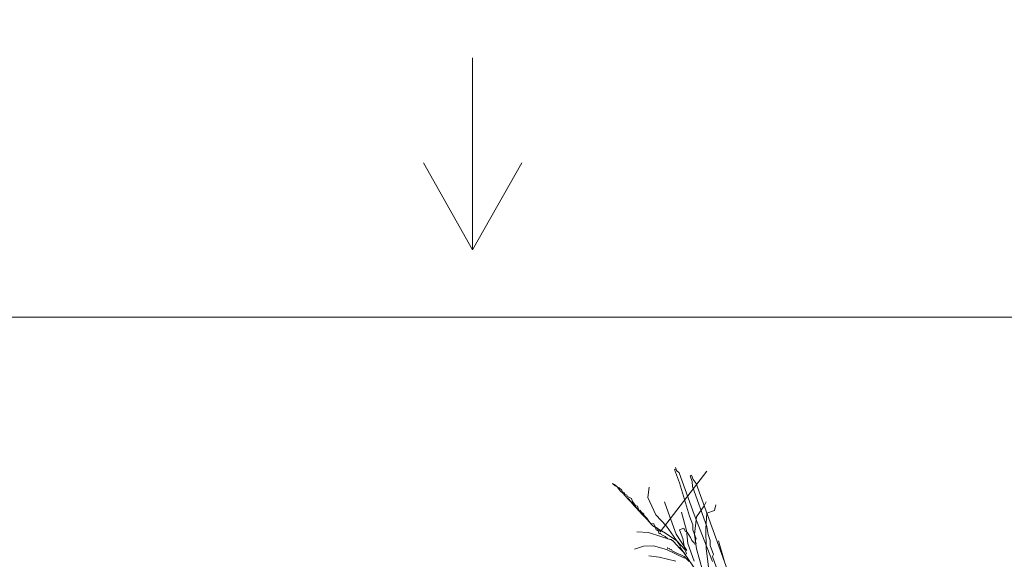
# Model space of a CAD drawing. Units: millimetres. Extents: x 595116 to 630915, y 909473 to 920225.
# Tile 39 of 134: x 629654.1 to 629671.98, y 919180.52 to 919190.32. Entities that reach past the tile are written whole.
import ezdxf

# ---------------------------------------------------------------- set-up
doc = ezdxf.new("R2010")
doc.units = ezdxf.units.MM
doc.layers.add('Dimension', color=3, linetype='Continuous', lineweight=18)
doc.layers.add('L-PLNT', color=85, linetype='Continuous', lineweight=13)
doc.styles.get("Standard").update_dxf_attribs({"font": 'arial.ttf'})
doc.dimstyles.new('ISO-25', dxfattribs={"dimtxt": 9, "dimasz": 6, "dimexe": 1.25, "dimexo": 0.625, "dimtad": 1, "dimlunit": 4, "dimtxsty": 'Standard', "dimcen": 2.5, "dimadec": 0, "dimazin": 0, "dimtfac": 1, "dimtmove": 0, "dimatfit": 3, "dimfxl": 1, "dimarcsym": 0})

# ---------------------------------------------------------------- blocks, each defined once
blk = doc.blocks.new('A$C4FB75ABC')
for p, q in [((2.2354, 4.7176), (2.2283, 4.715)), ((2.238, 4.7104), (2.2329, 4.7248)), ((2.2329, 4.7248), (2.2354, 4.7176)), ((2.1583, 4.4143), (2.3852, 4.7066)), ((2.2283, 4.715), (2.2515, 4.6504)), ((2.2504, 4.6987), (2.238, 4.7104)), ((2.3227, 4.4977), (2.2504, 4.6987)), ((2.3109, 4.688), (2.3037, 4.6854)), ((2.3037, 4.6854), (2.314, 4.6567)), ((2.3186, 4.6665), (2.3109, 4.688)), ((1.9382, 4.6431), (1.9285, 4.6477)), ((1.9285, 4.6477), (1.9408, 4.6359)), ((1.9506, 4.6313), (1.9382, 4.6431)), ((1.9408, 4.6359), (1.9506, 4.6313)), ((1.9603, 4.6267), (1.9506, 4.6313)), ((1.9506, 4.6313), (1.9655, 4.6124)), ((1.9726, 4.6149), (1.9603, 4.6267)), ((2.0989, 4.5793), (2.1049, 4.6301)), ((2.2515, 4.6504), (2.3011, 4.49)), ((2.314, 4.6567), (2.3146, 4.6326)), ((2.3146, 4.6326), (2.3843, 4.4389)), ((2.3336, 4.6475), (2.3186, 4.6665)), ((2.6279, 3.8295), (2.3336, 4.6475)), ((1.9655, 4.6124), (1.9778, 4.6006)), ((1.9752, 4.6078), (1.9726, 4.6149)), ((1.985, 4.6032), (1.9752, 4.6078)), ((1.9778, 4.6006), (2.0051, 4.5699)), ((1.9876, 4.596), (1.985, 4.6032)), ((1.9973, 4.5914), (1.9876, 4.596)), ((1.9999, 4.5842), (1.9973, 4.5914)), ((2.0097, 4.5796), (1.9999, 4.5842)), ((2.1238, 4.4424), (2.0025, 4.577)), ((2.0194, 4.575), (2.0097, 4.5796)), ((2.0246, 4.5607), (2.0194, 4.575)), ((2.137, 4.4958), (2.0989, 4.5793)), ((2.0051, 4.5699), (2.0174, 4.5581)), ((2.0174, 4.5581), (2.0323, 4.5391)), ((2.0395, 4.5417), (2.0246, 4.5607)), ((2.0323, 4.5391), (2.0447, 4.5274)), ((2.0493, 4.5371), (2.0395, 4.5417)), ((2.0447, 4.5274), (2.0719, 4.4967)), ((2.057, 4.5156), (2.0493, 4.5371)), ((2.197, 4.5092), (2.1789, 4.5595)), ((2.335, 4.486), (2.3723, 4.5399)), ((2.3723, 4.5399), (2.3815, 4.5594)), ((2.4211, 4.5169), (2.4277, 4.5436)), ((2.0642, 4.5182), (2.057, 4.5156)), ((2.0668, 4.511), (2.0642, 4.5182)), ((2.0791, 4.4992), (2.0668, 4.511)), ((2.0719, 4.4967), (2.0966, 4.4731)), ((2.0817, 4.4921), (2.0791, 4.4992)), ((2.094, 4.4803), (2.0817, 4.4921)), ((2.1115, 4.4542), (2.094, 4.4803)), ((2.189, 4.4415), (2.137, 4.4958)), ((2.2357, 4.4016), (2.197, 4.5092)), ((2.2859, 4.4197), (2.2621, 4.5084)), ((2.3011, 4.49), (2.3166, 4.4469)), ((2.4125, 4.2707), (2.3227, 4.4977)), ((2.325, 4.4013), (2.335, 4.486)), ((2.3797, 4.4291), (2.3852, 4.504)), ((2.3852, 4.504), (2.4211, 4.5169)), ((2.0966, 4.4731), (2.1115, 4.4542)), ((2.1238, 4.4424), (2.1115, 4.4542)), ((2.1115, 4.4542), (2.1284, 4.4522)), ((2.1336, 4.4378), (2.1238, 4.4424)), ((2.185, 4.4077), (2.1238, 4.4424)), ((2.1284, 4.4522), (2.1336, 4.4378)), ((2.1388, 4.4235), (2.1336, 4.4378)), ((2.1336, 4.4378), (2.1434, 4.4332)), ((2.1434, 4.4332), (2.1485, 4.4189)), ((2.2564, 4.3442), (2.189, 4.4415)), ((2.2736, 4.4314), (2.2521, 4.4237)), ((2.2788, 4.4171), (2.2736, 4.4314)), ((2.3166, 4.4469), (2.3172, 4.4228)), ((2.3843, 4.4389), (2.3901, 4.4004)), ((2.1029, 4.4105), (2.0449, 4.414)), ((2.222, 4.3723), (2.1029, 4.4105)), ((2.1485, 4.4189), (2.1388, 4.4235)), ((2.1485, 4.4189), (2.1557, 4.4214)), ((2.1537, 4.4045), (2.1485, 4.4189)), ((2.1609, 4.4071), (2.1537, 4.4045)), ((2.1557, 4.4214), (2.1583, 4.4143)), ((2.1634, 4.3999), (2.1609, 4.4071)), ((2.1829, 4.3907), (2.1634, 4.3999)), ((2.1953, 4.379), (2.1829, 4.3907)), ((2.2389, 4.3703), (2.185, 4.4077)), ((2.2882, 4.3232), (2.2357, 4.4016)), ((2.2521, 4.4237), (2.2676, 4.3807)), ((2.2885, 4.4125), (2.2788, 4.4171)), ((2.2922, 4.3571), (2.2859, 4.4197)), ((2.306, 4.3864), (2.2885, 4.4125)), ((2.3112, 4.372), (2.306, 4.3864)), ((2.3172, 4.4228), (2.3327, 4.3798)), ((2.3338, 4.3316), (2.325, 4.4013)), ((2.382, 4.3327), (2.3797, 4.4291)), ((2.3901, 4.4004), (2.4004, 4.3717)), ((2.0779, 4.3448), (2.0349, 4.3293)), ((2.1261, 4.346), (2.0779, 4.3448)), ((2.1893, 4.3282), (2.1261, 4.346)), ((2.1938, 4.3379), (2.1964, 4.3307)), ((2.2122, 4.3769), (2.1953, 4.379)), ((2.2245, 4.3652), (2.2122, 4.3769)), ((2.2518, 4.3344), (2.2245, 4.3652)), ((2.2785, 4.3278), (2.2389, 4.3703)), ((2.2538, 4.3417), (2.3557, 4.1924)), ((2.2676, 4.3807), (2.2759, 4.335)), ((2.3232, 4.271), (2.2922, 4.3571)), ((2.3235, 4.3603), (2.3112, 4.372)), ((2.3261, 4.3531), (2.3235, 4.3603)), ((2.3333, 4.3557), (2.3261, 4.3531)), ((2.3327, 4.3798), (2.3281, 4.37)), ((2.3281, 4.37), (2.3333, 4.3557)), ((2.4004, 4.3717), (2.401, 4.3476)), ((2.401, 4.3476), (2.4165, 4.3046)), ((2.4678, 4.2744), (2.4414, 4.3703)), ((2.154, 4.2911), (2.1032, 4.2972)), ((2.234, 4.2713), (2.154, 4.2911)), ((2.277, 4.2868), (2.1893, 4.3282)), ((2.1964, 4.3307), (2.2036, 4.3333)), ((2.2036, 4.3333), (2.2062, 4.3261)), ((2.2062, 4.3261), (2.2134, 4.3287)), ((2.2134, 4.3287), (2.2159, 4.3215)), ((2.2159, 4.3215), (2.2354, 4.3124)), ((2.2354, 4.3124), (2.2452, 4.3078)), ((2.2452, 4.3078), (2.255, 4.3032)), ((2.2641, 4.3227), (2.2518, 4.3344)), ((2.255, 4.3032), (2.2745, 4.294)), ((2.2765, 4.3109), (2.2641, 4.3227)), ((2.2745, 4.294), (2.2868, 4.2822)), ((2.2759, 4.335), (2.2862, 4.3063)), ((2.2791, 4.3037), (2.2765, 4.3109)), ((2.2862, 4.3063), (2.2791, 4.3037)), ((2.3628, 4.2285), (2.3338, 4.3316)), ((2.3941, 4.2317), (2.382, 4.3327)), ((2.4165, 4.3046), (2.4119, 4.2948)), ((2.4119, 4.2948), (2.43, 4.2446)), ((2.2868, 4.2822), (2.2991, 4.2704))]:
    blk.add_line(p, q)
blk = doc.blocks.new('LAWN-GRASS-TUFT')
blk.add_line((0.892, 3.485), (0.892, 0))
blk.add_lwpolyline([(0, 1.577), (0.892, 0), (1.785, 1.577)])
blk = doc.blocks.new('*D216')
at = {"layer": 'Defpoints', "color": 0, "transparency": 16777216}
for p in [(629743.541, 919411.928), (629505.041, 919411.828), (629743.541, 918832.378)]:
    blk.add_point(p, dxfattribs=at)
at = {"layer": 'Dimension', "color": 0, "lineweight": -2, "transparency": 16777216}
for p, q in [((629505.041, 919411.203), (629505.041, 918831.128)), ((629743.541, 919411.303), (629743.541, 918831.128)), ((629511.041, 918832.378), (629737.541, 918832.378))]:
    blk.add_line(p, q, dxfattribs=at)
at = {"layer": 'Dimension', "color": 0, "transparency": 16777216}
for points in [[(629511.041, 918833.378), (629511.041, 918831.378), (629505.041, 918832.378)], [(629737.541, 918833.378), (629737.541, 918831.378), (629743.541, 918832.378)]]:
    blk.add_solid(points, dxfattribs=at)
at = {"layer": 'Dimension', "color": 0, "transparency": 16777216, "insert": (629624.291, 918837.656), "char_height": 9, "attachment_point": 5}
blk.add_mtext('19\'-10 1/2"', dxfattribs=at)

msp = doc.modelspace()

# ---------------------------------------------------------------- linework, layer by layer
at = {"layer": 'L-PLNT'}
msp.add_line((629535.274, 919184.917), (629800.951, 919184.917), dxfattribs=at)

# ---------------------------------------------------------------- block references
msp.add_blockref('LAWN-GRASS-TUFT', (629661.43, 919186.14), dxfattribs=at)
at = {"layer": 'L-PLNT', "xscale": 3.753413438031968, "yscale": 3.753413438031968, "zscale": 3.753413438031968}
msp.add_blockref('A$C4FB75ABC', (629657.627, 919164.449), dxfattribs=at)

# ---------------------------------------------------------------- dimensions: what is measured, and where the dimension line sits
at = {"layer": 'Dimension'}
dim = msp.add_linear_dim(base=(629743.541, 918832.378), p1=(629505.041, 919411.828), p2=(629743.541, 919411.928), dimstyle='ISO-25', override={"dimdec": 1, "dimlfac": 1, "dimrnd": 0, "dimzin": 1, "dimdsep": 46, "dimlunit": 4, "dimfrac": 2}, dxfattribs=at)
dim.commit()
dim.dimension.update_dxf_attribs({"geometry": '*D216', "text_midpoint": (629624.291, 918837.656)})

doc.saveas('drawing.dxf')
